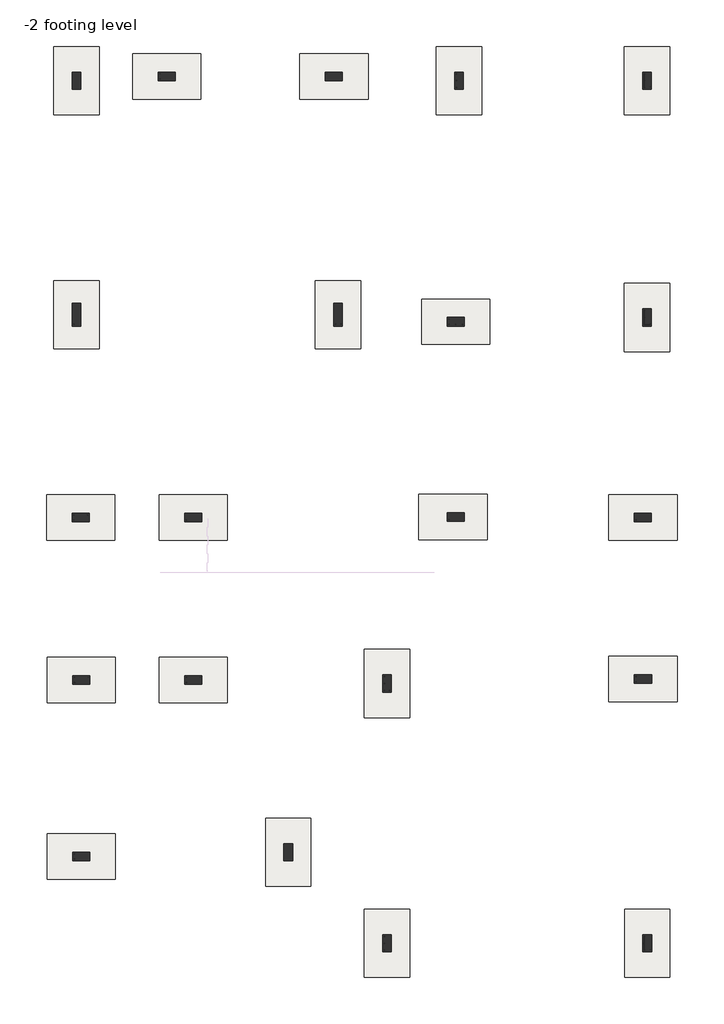
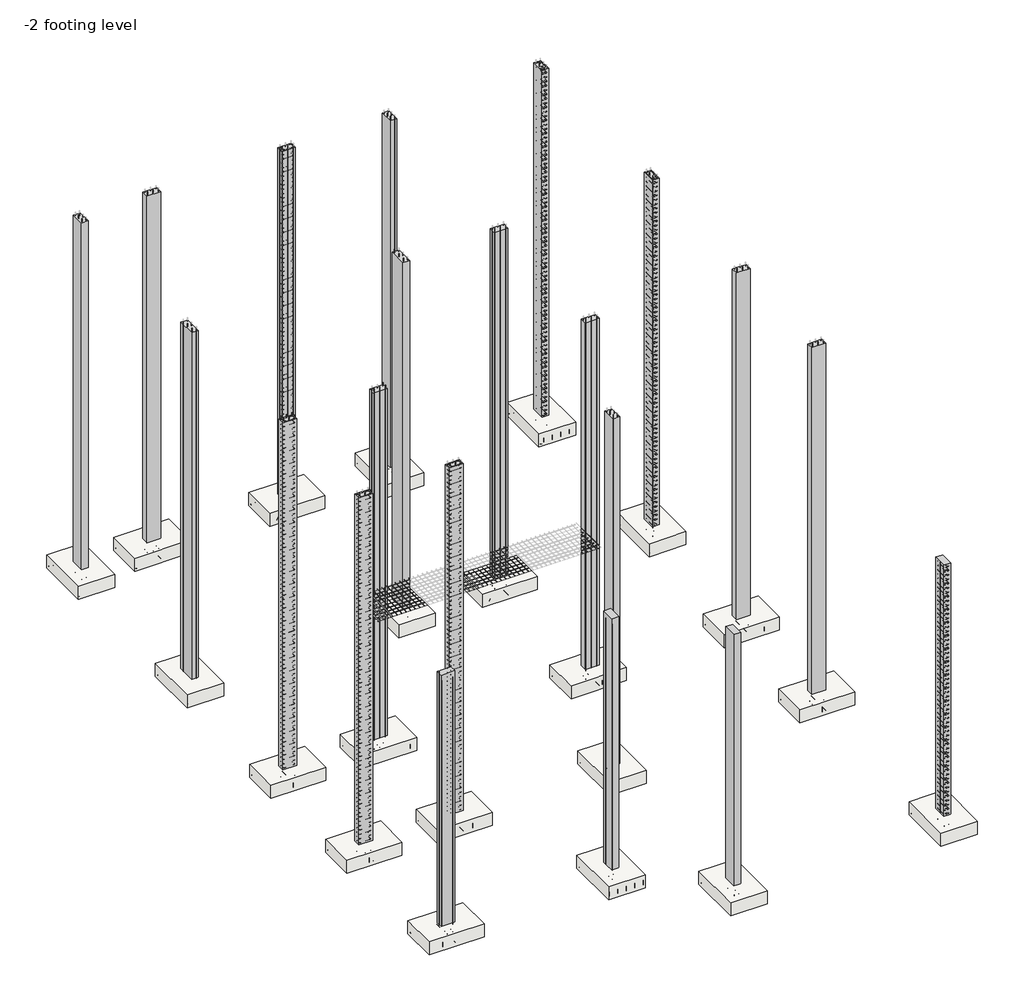
# One storey, part 1 of 9: 21 columns, 21 slabs.
"""IFC4 building model written with IfcOpenShell, lengths in millimetres."""

from ifc_helpers import new_model, si_unit, frame, origin, place, context, project, spatial, polyline, outline, extrude, faceted_brep, transform, mapped, element, save
from components import slab_5ba74754

model = new_model("IFC4")

# Units and contexts
model_context = context("Model", 3, world=origin())
ifc_project = project(units=[si_unit("LENGTHUNIT", "METRE", prefix="MILLI")], contexts=[model_context])

# Site, building, storey
site = spatial("IfcSite", under=ifc_project)
building = spatial("IfcBuilding", under=site)
storey = spatial("IfcBuildingStorey", under=building, Name="-2 footing level", Elevation=-1828.8)

# Columns
placement = place(None, origin())
element("IfcColumn", 1, ObjectType="Concrete-Rectangular-Column : 18.9", at=placement, inside=storey, context=model_context, shape_type="SweptSolid", body=[
    extrude(outline(polyline([(-8184.1001466, -7145.4266794), (-7726.9001466, -7145.4266794), (-7726.9001466, -7374.0266794), (-8184.1001466, -7374.0266794), (-8184.1001466, -7145.4266794)])), frame((0.0, 0.0, -1828.8), z_axis=(0.0, 0.0, 1.0), x_axis=(1.0, 0.0, 0.0)), (0.0, 0.0, 1.0), 8839.2),
])
element("IfcColumn", 2, ObjectType="Concrete-Rectangular-Column : 18.9", at=placement, inside=storey, context=model_context, shape_type="Brep", body=[
    faceted_brep([(-2287.8823872, -6916.8266794, -1828.8), (-2287.8823872, -7374.0266794, -1828.8), (-2516.4823872, -7374.0266794, -1828.8), (-2516.4823872, -6916.8266794, -1828.8), (-2287.8823872, -6916.8266794, 7010.4), (-2287.8823872, -7374.0266794, 7010.4), (-2287.8823872, -7374.0266794, 6553.2), (-2287.8823872, -7374.0266794, 3505.2), (-2287.8823872, -7374.0266794, 3048.0), (-2287.8823872, -6916.8266794, 3048.0), (-2287.8823872, -6916.8266794, 3505.2), (-2287.8823872, -6916.8266794, 6553.2), (-2516.4823872, -7374.0266794, 7010.4), (-2516.4823872, -7374.0266794, 6553.2), (-2516.4823872, -7374.0266794, 3505.2), (-2516.4823872, -7374.0266794, 3048.0), (-2516.4823872, -6916.8266794, 7010.4), (-2516.4823872, -6916.8266794, 6553.2), (-2516.4823872, -6916.8266794, 3505.2), (-2516.4823872, -6916.8266794, 3048.0)], [[[0, 1, 2, 3]], [[4, 5, 6, 7, 8, 1, 0, 9, 10, 11]], [[5, 12, 13, 14, 15, 2, 1, 8, 7, 6]], [[12, 16, 17, 18, 19, 3, 2, 15, 14, 13]], [[16, 4, 11, 10, 9, 0, 3, 19, 18, 17]], [[4, 16, 12, 5]]]),
])
element("IfcColumn", 3, ObjectType="Concrete-Rectangular-Column : 18.9", at=placement, inside=storey, context=model_context, shape_type="SweptSolid", body=[
    extrude(outline(polyline([(358.2588295, -9362.9794723), (358.2588295, -9820.1794723), (129.6588295, -9820.1794723), (129.6588295, -9362.9794723), (358.2588295, -9362.9794723)])), frame((0.0, 0.0, -1828.8), z_axis=(0.0, 0.0, 1.0), x_axis=(1.0, 0.0, 0.0)), (0.0, 0.0, 1.0), 8839.2),
])
element("IfcColumn", 4, ObjectType="Concrete-Rectangular-Column : 18.9", at=placement, inside=storey, context=model_context, shape_type="SweptSolid", body=[
    extrude(outline(polyline([(7338.2179176, -9362.9794723), (7338.2179176, -9820.1794723), (7109.6179176, -9820.1794723), (7109.6179176, -9362.9794723), (7338.2179176, -9362.9794723)])), frame((0.0, 0.0, -1828.8), z_axis=(0.0, 0.0, 1.0), x_axis=(1.0, 0.0, 0.0)), (0.0, 0.0, 1.0), 8839.2),
])
element("IfcColumn", 5, ObjectType="Concrete-Rectangular-Column : 18.9", at=placement, inside=storey, context=model_context, shape_type="Brep", body=[
    faceted_brep([(6881.0179176, -2394.7351307, -1828.8), (7338.2179176, -2394.7351307, -1828.8), (7338.2179176, -2623.3351307, -1828.8), (6881.0179176, -2623.3351307, -1828.8), (6881.0179176, -2394.7351307, 10363.2), (7338.2179176, -2394.7351307, 10363.2), (7338.2179176, -2394.7351307, 10058.4), (7338.2179176, -2394.7351307, 7010.4), (7338.2179176, -2394.7351307, 6553.2), (7338.2179176, -2394.7351307, 3505.2), (7338.2179176, -2394.7351307, 3048.0), (7338.2179176, -2394.7351307, 0.0), (7338.2179176, -2394.7351307, -609.6), (6881.0179176, -2394.7351307, -609.6), (6881.0179176, -2394.7351307, 0.0), (6881.0179176, -2394.7351307, 3048.0), (6881.0179176, -2394.7351307, 3505.2), (6881.0179176, -2394.7351307, 6553.2), (6881.0179176, -2394.7351307, 7010.4), (6881.0179176, -2394.7351307, 10058.4), (7338.2179176, -2623.3351307, 10363.2), (7338.2179176, -2623.3351307, 10058.4), (7338.2179176, -2623.3351307, 7010.4), (7338.2179176, -2623.3351307, 6553.2), (7338.2179176, -2623.3351307, 3505.2), (7338.2179176, -2623.3351307, 3048.0), (7338.2179176, -2623.3351307, 0.0), (7338.2179176, -2623.3351307, -609.6), (6881.0179176, -2623.3351307, 10363.2), (6881.0179176, -2623.3351307, 10058.4)], [[[0, 1, 2, 3]], [[4, 5, 6, 7, 8, 9, 10, 11, 12, 1, 0, 13, 14, 15, 16, 17, 18, 19]], [[5, 20, 21, 22, 23, 24, 25, 26, 27, 2, 1, 12, 11, 10, 9, 8, 7, 6]], [[20, 28, 29, 3, 2, 27, 26, 25, 24, 23, 22, 21]], [[28, 4, 19, 18, 17, 16, 15, 14, 13, 0, 3, 29]], [[4, 28, 20, 5]]]),
])
element("IfcColumn", 6, ObjectType="Concrete-Rectangular-Column : 18.9", at=placement, inside=storey, context=model_context, shape_type="Brep", body=[
    faceted_brep([(129.6588295, -2851.9351307, -1828.8), (129.6588295, -2394.7351307, -1828.8), (358.2588295, -2394.7351307, -1828.8), (358.2588295, -2851.9351307, -1828.8), (129.6588295, -2851.9351307, 10363.2), (129.6588295, -2394.7351307, 10363.2), (129.6588295, -2394.7351307, 10058.4), (129.6588295, -2394.7351307, 7010.4), (129.6588295, -2394.7351307, 6553.2), (129.6588295, -2394.7351307, 3505.2), (129.6588295, -2394.7351307, 3048.0), (129.6588295, -2394.7351307, 0.0), (129.6588295, -2394.7351307, -609.6), (129.6588295, -2851.9351307, -609.6), (129.6588295, -2851.9351307, 0.0), (129.6588295, -2851.9351307, 3048.0), (129.6588295, -2851.9351307, 3505.2), (129.6588295, -2851.9351307, 6553.2), (129.6588295, -2851.9351307, 7010.4), (129.6588295, -2851.9351307, 10058.4), (358.2588295, -2394.7351307, 10363.2), (358.2588295, -2394.7351307, 10058.4), (358.2588295, -2394.7351307, 7010.4), (358.2588295, -2394.7351307, 6553.2), (358.2588295, -2394.7351307, 3505.2), (358.2588295, -2394.7351307, 3048.0), (358.2588295, -2394.7351307, 0.0), (358.2588295, -2394.7351307, -609.6), (358.2588295, -2851.9351307, 10363.2), (358.2588295, -2851.9351307, 10058.4), (358.2588295, -2851.9351307, 7010.4), (358.2588295, -2851.9351307, 6553.2), (358.2588295, -2851.9351307, 3505.2), (358.2588295, -2851.9351307, 3048.0), (358.2588295, -2851.9351307, 0.0), (358.2588295, -2851.9351307, -609.6)], [[[0, 1, 2, 3]], [[4, 5, 6, 7, 8, 9, 10, 11, 12, 1, 0, 13, 14, 15, 16, 17, 18, 19]], [[5, 20, 21, 22, 23, 24, 25, 26, 27, 2, 1, 12, 11, 10, 9, 8, 7, 6]], [[20, 28, 29, 30, 31, 32, 33, 34, 35, 3, 2, 27, 26, 25, 24, 23, 22, 21]], [[28, 4, 19, 18, 17, 16, 15, 14, 13, 0, 3, 35, 34, 33, 32, 31, 30, 29]], [[4, 28, 20, 5]]]),
])
element("IfcColumn", 7, ObjectType="Concrete-Rectangular-Column : 18.9", at=placement, inside=storey, context=model_context, shape_type="Brep", body=[
    faceted_brep([(-4721.8698352, -2640.4945725, -1828.8), (-5179.0698352, -2640.4945725, -1828.8), (-5179.0698352, -2411.8945725, -1828.8), (-4721.8698352, -2411.8945725, -1828.8), (-4721.8698352, -2640.4945725, 10363.2), (-5179.0698352, -2640.4945725, 10363.2), (-5179.0698352, -2640.4945725, 10058.4), (-5179.0698352, -2640.4945725, 7010.4), (-5179.0698352, -2640.4945725, 6553.2), (-5179.0698352, -2640.4945725, 3505.2), (-5179.0698352, -2640.4945725, 3048.0), (-5179.0698352, -2640.4945725, 0.0), (-5179.0698352, -2640.4945725, -609.6), (-4721.8698352, -2640.4945725, -609.6), (-4721.8698352, -2640.4945725, 0.0), (-4721.8698352, -2640.4945725, 3048.0), (-4721.8698352, -2640.4945725, 3505.2), (-4721.8698352, -2640.4945725, 6553.2), (-4721.8698352, -2640.4945725, 7010.4), (-4721.8698352, -2640.4945725, 10058.4), (-5179.0698352, -2411.8945725, 10363.2), (-5179.0698352, -2411.8945725, 10058.4), (-5179.0698352, -2411.8945725, 7010.4), (-5179.0698352, -2411.8945725, 6553.2), (-5179.0698352, -2411.8945725, 3505.2), (-5179.0698352, -2411.8945725, 3048.0), (-5179.0698352, -2411.8945725, 0.0), (-5179.0698352, -2411.8945725, -609.6), (-4721.8698352, -2411.8945725, 10363.2), (-4721.8698352, -2411.8945725, 10058.4), (-4721.8698352, -2411.8945725, 7010.4), (-4721.8698352, -2411.8945725, 6553.2), (-4721.8698352, -2411.8945725, 3505.2), (-4721.8698352, -2411.8945725, 3048.0), (-4721.8698352, -2411.8945725, 0.0), (-4721.8698352, -2411.8945725, -609.6)], [[[0, 1, 2, 3]], [[4, 5, 6, 7, 8, 9, 10, 11, 12, 1, 0, 13, 14, 15, 16, 17, 18, 19]], [[5, 20, 21, 22, 23, 24, 25, 26, 27, 2, 1, 12, 11, 10, 9, 8, 7, 6]], [[20, 28, 29, 30, 31, 32, 33, 34, 35, 3, 2, 27, 26, 25, 24, 23, 22, 21]], [[28, 4, 19, 18, 17, 16, 15, 14, 13, 0, 3, 35, 34, 33, 32, 31, 30, 29]], [[4, 28, 20, 5]]]),
])
element("IfcColumn", 8, ObjectType="Concrete-Rectangular-Column : 18.9", at=placement, inside=storey, context=model_context, shape_type="Brep", body=[
    faceted_brep([(-7726.9001466, -2640.4945725, -1828.8), (-8184.1001466, -2640.4945725, -1828.8), (-8184.1001466, -2411.8945725, -1828.8), (-7726.9001466, -2411.8945725, -1828.8), (-7726.9001466, -2640.4945725, 10363.2), (-8184.1001466, -2640.4945725, 10363.2), (-8184.1001466, -2640.4945725, 10058.4), (-8184.1001466, -2640.4945725, 7010.4), (-8184.1001466, -2640.4945725, 6553.2), (-8184.1001466, -2640.4945725, 3505.2), (-8184.1001466, -2640.4945725, 3048.0), (-7726.9001466, -2640.4945725, 3048.0), (-7726.9001466, -2640.4945725, 3505.2), (-7726.9001466, -2640.4945725, 6553.2), (-7726.9001466, -2640.4945725, 7010.4), (-7726.9001466, -2640.4945725, 10058.4), (-8184.1001466, -2411.8945725, 10363.2), (-8184.1001466, -2411.8945725, 10058.4), (-8184.1001466, -2411.8945725, 7010.4), (-8184.1001466, -2411.8945725, 6553.2), (-8184.1001466, -2411.8945725, 3505.2), (-8184.1001466, -2411.8945725, 3048.0), (-7726.9001466, -2411.8945725, 10363.2), (-7726.9001466, -2411.8945725, 10058.4), (-7726.9001466, -2411.8945725, 7010.4), (-7726.9001466, -2411.8945725, 6553.2), (-7726.9001466, -2411.8945725, 3505.2), (-7726.9001466, -2411.8945725, 3048.0)], [[[0, 1, 2, 3]], [[4, 5, 6, 7, 8, 9, 10, 1, 0, 11, 12, 13, 14, 15]], [[5, 16, 17, 18, 19, 20, 21, 2, 1, 10, 9, 8, 7, 6]], [[16, 22, 23, 24, 25, 26, 27, 3, 2, 21, 20, 19, 18, 17]], [[22, 4, 15, 14, 13, 12, 11, 0, 3, 27, 26, 25, 24, 23]], [[4, 22, 16, 5]]]),
])
element("IfcColumn", 9, ObjectType="Concrete-Rectangular-Column : 18.9", at=placement, inside=storey, context=model_context, shape_type="Brep", body=[
    faceted_brep([(-4722.5687565, 1710.0401753, -1828.8), (-5179.7687565, 1710.0401753, -1828.8), (-5179.7687565, 1938.6401753, -1828.8), (-4722.5687565, 1938.6401753, -1828.8), (-4722.5687565, 1710.0401753, 10363.2), (-5179.0698352, 1710.0401753, 10363.2), (-5179.7687565, 1710.0401753, 10363.2), (-4722.5687565, 1710.0401753, 10058.4), (-5179.7687565, 1722.9180142, 10363.2), (-5179.7687565, 1938.6401753, 10363.2), (-5179.7687565, 1938.6401753, 10058.4), (-5179.7687565, 1938.6401753, 7010.4), (-5179.7687565, 1938.6401753, 6553.2), (-5179.7687565, 1938.6401753, 3505.2), (-5179.7687565, 1938.6401753, 3048.0), (-5179.7687565, 1938.6401753, 0.0), (-5179.7687565, 1938.6401753, -609.6), (-4722.5687565, 1938.6401753, 10363.2), (-4722.5687565, 1938.6401753, 10058.4), (-4722.5687565, 1938.6401753, 7010.4), (-4722.5687565, 1938.6401753, 6553.2), (-4722.5687565, 1938.6401753, 3505.2), (-4722.5687565, 1938.6401753, 3048.0), (-4722.5687565, 1938.6401753, 0.0), (-4722.5687565, 1938.6401753, -609.6), (-4722.5687565, 1722.9180142, 10363.2)], [[[0, 1, 2, 3]], [[4, 5, 6, 1, 0, 7]], [[6, 8, 9, 10, 11, 12, 13, 14, 15, 16, 2, 1]], [[9, 17, 18, 19, 20, 21, 22, 23, 24, 3, 2, 16, 15, 14, 13, 12, 11, 10]], [[17, 25, 4, 7, 0, 3, 24, 23, 22, 21, 20, 19, 18]], [[4, 25, 17, 9, 8, 6, 5]]]),
])
element("IfcColumn", 10, ObjectType="Concrete-Rectangular-Column : 18.9", at=placement, inside=storey, context=model_context, shape_type="Brep", body=[
    faceted_brep([(-7740.635762, 1710.0401753, -1828.8), (-8197.835762, 1710.0401753, -1828.8), (-8197.835762, 1938.6401753, -1828.8), (-7740.635762, 1938.6401753, -1828.8), (-7740.635762, 1710.0401753, 10363.2), (-8197.835762, 1710.0401753, 10363.2), (-8197.835762, 1710.0401753, 10058.4), (-7740.635762, 1710.0401753, 10058.4), (-8197.835762, 1938.6401753, 10363.2), (-8197.835762, 1938.6401753, 10058.4), (-7740.635762, 1938.6401753, 10363.2), (-7740.635762, 1938.6401753, 10058.4)], [[[0, 1, 2, 3]], [[4, 5, 6, 1, 0, 7]], [[5, 8, 9, 2, 1, 6]], [[8, 10, 11, 3, 2, 9]], [[10, 4, 7, 0, 3, 11]], [[4, 10, 8, 5]]]),
])
element("IfcColumn", 11, ObjectType="Concrete-Rectangular-Column : 18.9", at=placement, inside=storey, context=model_context, shape_type="Brep", body=[
    faceted_brep([(1859.2315874, 7190.7340845, -1828.8), (2316.4315874, 7190.7340845, -1828.8), (2316.4315874, 6962.1340845, -1828.8), (1859.2315874, 6962.1340845, -1828.8), (1859.2315874, 7190.7340845, 10363.2), (2316.4315874, 7190.7340845, 10363.2), (2316.4315874, 7190.7340845, 10058.4), (2316.4315874, 7190.7340845, 7010.4), (2316.4315874, 7190.7340845, 6553.2), (2316.4315874, 7190.7340845, 3505.2), (2316.4315874, 7190.7340845, 3048.0), (2316.4315874, 7190.7340845, 0.0), (2316.4315874, 7190.7340845, -609.6), (1859.2315874, 7190.7340845, -609.6), (1859.2315874, 7190.7340845, 0.0), (1859.2315874, 7190.7340845, 3048.0), (1859.2315874, 7190.7340845, 3505.2), (1859.2315874, 7190.7340845, 6553.2), (1859.2315874, 7190.7340845, 7010.4), (1859.2315874, 7190.7340845, 10058.4), (2316.4315874, 6962.1340845, 10363.2), (2316.4315874, 6962.1340845, 10058.4), (2316.4315874, 6962.1340845, 7010.4), (2316.4315874, 6962.1340845, 6553.2), (2316.4315874, 6962.1340845, 3505.2), (2316.4315874, 6962.1340845, 3048.0), (2316.4315874, 6962.1340845, 0.0), (2316.4315874, 6962.1340845, -609.6), (1859.2315874, 6962.1340845, 10363.2), (1859.2315874, 6962.1340845, 10058.4), (1859.2315874, 6962.1340845, 7010.4), (1859.2315874, 6962.1340845, 6553.2), (1859.2315874, 6962.1340845, 3505.2), (1859.2315874, 6962.1340845, 3048.0), (1859.2315874, 6962.1340845, 0.0), (1859.2315874, 6962.1340845, -609.6)], [[[0, 1, 2, 3]], [[4, 5, 6, 7, 8, 9, 10, 11, 12, 1, 0, 13, 14, 15, 16, 17, 18, 19]], [[5, 20, 21, 22, 23, 24, 25, 26, 27, 2, 1, 12, 11, 10, 9, 8, 7, 6]], [[20, 28, 29, 30, 31, 32, 33, 34, 35, 3, 2, 27, 26, 25, 24, 23, 22, 21]], [[28, 4, 19, 18, 17, 16, 15, 14, 13, 0, 3, 35, 34, 33, 32, 31, 30, 29]], [[4, 28, 20, 5]]]),
])
element("IfcColumn", 12, ObjectType="Concrete-Rectangular-Column : 18.9", at=placement, inside=storey, context=model_context, shape_type="Brep", body=[
    faceted_brep([(7108.8638577, 6962.1340845, -1828.8), (7108.8638577, 7419.3340845, -1828.8), (7337.4638577, 7419.3340845, -1828.8), (7337.4638577, 6962.1340845, -1828.8), (7108.8638577, 6962.1340845, 10363.2), (7108.8638577, 7419.3340845, 10363.2), (7108.8638577, 7419.3340845, 10058.4), (7108.8638577, 6962.1340845, 10058.4), (7337.4638577, 7419.3340845, 10363.2), (7337.4638577, 7419.3340845, 10058.4), (7337.4638577, 6962.1340845, 10363.2), (7337.4638577, 6962.1340845, 10058.4)], [[[0, 1, 2, 3]], [[4, 5, 6, 1, 0, 7]], [[5, 8, 9, 2, 1, 6]], [[8, 10, 11, 3, 2, 9]], [[10, 4, 7, 0, 3, 11]], [[4, 10, 8, 5]]]),
])
element("IfcColumn", 13, ObjectType="Concrete-Rectangular-Column : 18.9", at=placement, inside=storey, context=model_context, shape_type="Brep", body=[
    faceted_brep([(2316.4315874, 1722.9180142, -1828.8), (1859.2315874, 1722.9180142, -1828.8), (1859.2315874, 1951.5180142, -1828.8), (2316.4315874, 1951.5180142, -1828.8), (2316.4315874, 1722.9180142, 10363.2), (1859.2315874, 1722.9180142, 10363.2), (1859.2315874, 1722.9180142, 10058.4), (1859.2315874, 1722.9180142, 7010.4), (1859.2315874, 1722.9180142, 6553.2), (1859.2315874, 1722.9180142, 3505.2), (1859.2315874, 1722.9180142, 3048.0), (1859.2315874, 1722.9180142, 0.0), (1859.2315874, 1722.9180142, -609.6), (2316.4315874, 1722.9180142, -609.6), (2316.4315874, 1722.9180142, 0.0), (2316.4315874, 1722.9180142, 3048.0), (2316.4315874, 1722.9180142, 3505.2), (2316.4315874, 1722.9180142, 6553.2), (2316.4315874, 1722.9180142, 7010.4), (2316.4315874, 1722.9180142, 10058.4), (1859.2315874, 1951.5180142, 10363.2), (1859.2315874, 1951.5180142, 10058.4), (1859.2315874, 1951.5180142, 7010.4), (1859.2315874, 1951.5180142, 6553.2), (1859.2315874, 1951.5180142, 3505.2), (1859.2315874, 1951.5180142, 3048.0), (1859.2315874, 1951.5180142, 0.0), (1859.2315874, 1951.5180142, -609.6), (2316.4315874, 1951.5180142, 10363.2), (2316.4315874, 1951.5180142, 10058.4), (2316.4315874, 1951.5180142, 7010.4), (2316.4315874, 1951.5180142, 6553.2), (2316.4315874, 1951.5180142, 3505.2), (2316.4315874, 1951.5180142, 3048.0), (2316.4315874, 1951.5180142, 0.0), (2316.4315874, 1951.5180142, -609.6)], [[[0, 1, 2, 3]], [[4, 5, 6, 7, 8, 9, 10, 11, 12, 1, 0, 13, 14, 15, 16, 17, 18, 19]], [[5, 20, 21, 22, 23, 24, 25, 26, 27, 2, 1, 12, 11, 10, 9, 8, 7, 6]], [[20, 28, 29, 30, 31, 32, 33, 34, 35, 3, 2, 27, 26, 25, 24, 23, 22, 21]], [[28, 4, 19, 18, 17, 16, 15, 14, 13, 0, 3, 35, 34, 33, 32, 31, 30, 29]], [[4, 28, 20, 5]]]),
])
element("IfcColumn", 14, ObjectType="Concrete-Rectangular-Column : 18.9", at=placement, inside=storey, context=model_context, shape_type="Brep", body=[
    faceted_brep([(7336.8310303, 1718.3038411, -1828.8), (6879.6310303, 1718.3038411, -1828.8), (6879.6310303, 1946.9038411, -1828.8), (7336.8310303, 1946.9038411, -1828.8), (7336.8310303, 1718.3038411, 10363.2), (6994.5638577, 1718.3038411, 10363.2), (6879.6310303, 1718.3038411, 10363.2), (7336.8310303, 1718.3038411, -609.6), (7336.8310303, 1718.3038411, 0.0), (7336.8310303, 1718.3038411, 3048.0), (7336.8310303, 1718.3038411, 3505.2), (7336.8310303, 1718.3038411, 6553.2), (7336.8310303, 1718.3038411, 7010.4), (7336.8310303, 1718.3038411, 10058.4), (6879.6310303, 1722.9180142, 10363.2), (6879.6310303, 1946.9038411, 10363.2), (6879.6310303, 1946.9038411, 10058.4), (6994.5638577, 1946.9038411, 10363.2), (7336.8310303, 1946.9038411, 10363.2), (7336.8310303, 1946.9038411, 10058.4), (7336.8310303, 1946.9038411, 7010.4), (7336.8310303, 1946.9038411, 6553.2), (7336.8310303, 1946.9038411, 3505.2), (7336.8310303, 1946.9038411, 3048.0), (7336.8310303, 1946.9038411, 0.0), (7336.8310303, 1946.9038411, -609.6)], [[[0, 1, 2, 3]], [[4, 5, 6, 1, 0, 7, 8, 9, 10, 11, 12, 13]], [[6, 14, 15, 16, 2, 1]], [[15, 17, 18, 19, 20, 21, 22, 23, 24, 25, 3, 2, 16]], [[18, 4, 13, 12, 11, 10, 9, 8, 7, 0, 3, 25, 24, 23, 22, 21, 20, 19]], [[4, 18, 17, 15, 14, 6, 5]]]),
])
element("IfcColumn", 15, ObjectType="Concrete-Rectangular-Column : 18.9", at=placement, inside=storey, context=model_context, shape_type="Brep", body=[
    faceted_brep([(2290.2821988, 13770.1951007, -1828.8), (2290.2821988, 13312.9951007, -1828.8), (2061.6821988, 13312.9951007, -1828.8), (2061.6821988, 13770.1951007, -1828.8), (2290.2821988, 13770.1951007, 10363.2), (2290.2821988, 13312.9951007, 10363.2), (2290.2821988, 13312.9951007, 10058.4), (2290.2821988, 13312.9951007, 7010.4), (2290.2821988, 13312.9951007, 6553.2), (2290.2821988, 13312.9951007, 3505.2), (2290.2821988, 13312.9951007, 3048.0), (2290.2821988, 13312.9951007, 0.0), (2290.2821988, 13312.9951007, -609.6), (2290.2821988, 13770.1951007, -609.6), (2290.2821988, 13770.1951007, 0.0), (2290.2821988, 13770.1951007, 3048.0), (2290.2821988, 13770.1951007, 3505.2), (2290.2821988, 13770.1951007, 6553.2), (2290.2821988, 13770.1951007, 7010.4), (2290.2821988, 13770.1951007, 10058.4), (2061.6821988, 13312.9951007, 10363.2), (2061.6821988, 13312.9951007, 10058.4), (2061.6821988, 13312.9951007, 7010.4), (2061.6821988, 13312.9951007, 6553.2), (2061.6821988, 13312.9951007, 3505.2), (2061.6821988, 13312.9951007, 3048.0), (2061.6821988, 13312.9951007, 0.0), (2061.6821988, 13312.9951007, -609.6), (2061.6821988, 13770.1951007, 10363.2), (2061.6821988, 13770.1951007, 10058.4), (2061.6821988, 13770.1951007, 7010.4), (2061.6821988, 13770.1951007, 6553.2), (2061.6821988, 13770.1951007, 3505.2), (2061.6821988, 13770.1951007, 3048.0), (2061.6821988, 13770.1951007, 0.0), (2061.6821988, 13770.1951007, -609.6)], [[[0, 1, 2, 3]], [[4, 5, 6, 7, 8, 9, 10, 11, 12, 1, 0, 13, 14, 15, 16, 17, 18, 19]], [[5, 20, 21, 22, 23, 24, 25, 26, 27, 2, 1, 12, 11, 10, 9, 8, 7, 6]], [[20, 28, 29, 30, 31, 32, 33, 34, 35, 3, 2, 27, 26, 25, 24, 23, 22, 21]], [[28, 4, 19, 18, 17, 16, 15, 14, 13, 0, 3, 35, 34, 33, 32, 31, 30, 29]], [[4, 28, 20, 5]]]),
])
element("IfcColumn", 16, ObjectType="Concrete-Rectangular-Column : 18.9", at=placement, inside=storey, context=model_context, shape_type="Brep", body=[
    faceted_brep([(7337.4638577, 13770.1951007, -1828.8), (7337.4638577, 13312.9951007, -1828.8), (7108.8638577, 13312.9951007, -1828.8), (7108.8638577, 13770.1951007, -1828.8), (7337.4638577, 13770.1951007, 10363.2), (7337.4638577, 13312.9951007, 10363.2), (7337.4638577, 13312.9951007, 10058.4), (7337.4638577, 13770.1951007, 10058.4), (7108.8638577, 13312.9951007, 10363.2), (7108.8638577, 13312.9951007, 10058.4), (7108.8638577, 13770.1951007, 10363.2), (7108.8638577, 13770.1951007, 10058.4)], [[[0, 1, 2, 3]], [[4, 5, 6, 1, 0, 7]], [[5, 8, 9, 2, 1, 6]], [[8, 10, 11, 3, 2, 9]], [[10, 4, 7, 0, 3, 11]], [[4, 10, 8, 5]]]),
])
element("IfcColumn", 17, ObjectType="Concrete-Rectangular-Column : 18.9", at=placement, inside=storey, context=model_context, shape_type="Brep", body=[
    faceted_brep([(-1405.4178012, 13770.1951007, -1828.8), (-948.2178012, 13770.1951007, -1828.8), (-948.2178012, 13541.5951007, -1828.8), (-1405.4178012, 13541.5951007, -1828.8), (-1405.4178012, 13770.1951007, 10363.2), (-948.2178012, 13770.1951007, 10363.2), (-948.2178012, 13770.1951007, 10058.4), (-948.2178012, 13770.1951007, 7010.4), (-948.2178012, 13770.1951007, 6553.2), (-948.2178012, 13770.1951007, 3505.2), (-948.2178012, 13770.1951007, 3048.0), (-948.2178012, 13770.1951007, 0.0), (-948.2178012, 13770.1951007, -609.6), (-1405.4178012, 13770.1951007, -609.6), (-1405.4178012, 13770.1951007, 0.0), (-1405.4178012, 13770.1951007, 3048.0), (-1405.4178012, 13770.1951007, 3505.2), (-1405.4178012, 13770.1951007, 6553.2), (-1405.4178012, 13770.1951007, 7010.4), (-1405.4178012, 13770.1951007, 10058.4), (-948.2178012, 13541.5951007, 10363.2), (-948.2178012, 13541.5951007, 10058.4), (-948.2178012, 13541.5951007, 7010.4), (-948.2178012, 13541.5951007, 6553.2), (-948.2178012, 13541.5951007, 3505.2), (-948.2178012, 13541.5951007, 3048.0), (-948.2178012, 13541.5951007, 0.0), (-948.2178012, 13541.5951007, -609.6), (-1405.4178012, 13541.5951007, 10363.2), (-1405.4178012, 13541.5951007, 10058.4), (-1405.4178012, 13541.5951007, 7010.4), (-1405.4178012, 13541.5951007, 6553.2), (-1405.4178012, 13541.5951007, 3505.2), (-1405.4178012, 13541.5951007, 3048.0), (-1405.4178012, 13541.5951007, 0.0), (-1405.4178012, 13541.5951007, -609.6)], [[[0, 1, 2, 3]], [[4, 5, 6, 7, 8, 9, 10, 11, 12, 1, 0, 13, 14, 15, 16, 17, 18, 19]], [[5, 20, 21, 22, 23, 24, 25, 26, 27, 2, 1, 12, 11, 10, 9, 8, 7, 6]], [[20, 28, 29, 30, 31, 32, 33, 34, 35, 3, 2, 27, 26, 25, 24, 23, 22, 21]], [[28, 4, 19, 18, 17, 16, 15, 14, 13, 0, 3, 35, 34, 33, 32, 31, 30, 29]], [[4, 28, 20, 5]]]),
])
element("IfcColumn", 18, ObjectType="Concrete-Rectangular-Column : 18.9", at=placement, inside=storey, context=model_context, shape_type="Brep", body=[
    faceted_brep([(-5887.9819615, 13770.1951007, -1828.8), (-5430.7819615, 13770.1951007, -1828.8), (-5430.7819615, 13541.5951007, -1828.8), (-5887.9819615, 13541.5951007, -1828.8), (-5887.9819615, 13770.1951007, 10363.2), (-5430.7819615, 13770.1951007, 10363.2), (-5430.7819615, 13770.1951007, 10058.4), (-5430.7819615, 13770.1951007, 7010.4), (-5430.7819615, 13770.1951007, 6553.2), (-5430.7819615, 13770.1951007, 3352.8), (-5430.7819615, 13770.1951007, 3048.0), (-5430.7819615, 13770.1951007, 0.0), (-5430.7819615, 13770.1951007, -609.6), (-5887.9819615, 13770.1951007, -609.6), (-5887.9819615, 13770.1951007, 0.0), (-5887.9819615, 13770.1951007, 3048.0), (-5887.9819615, 13770.1951007, 3352.8), (-5887.9819615, 13770.1951007, 6553.2), (-5887.9819615, 13770.1951007, 7010.4), (-5887.9819615, 13770.1951007, 10058.4), (-5430.7819615, 13541.5951007, 10363.2), (-5430.7819615, 13541.5951007, 10058.4), (-5430.7819615, 13541.5951007, 7010.4), (-5430.7819615, 13541.5951007, 6553.2), (-5430.7819615, 13541.5951007, 3352.8), (-5430.7819615, 13541.5951007, 3048.0), (-5430.7819615, 13541.5951007, 0.0), (-5430.7819615, 13541.5951007, -609.6), (-5887.9819615, 13541.5951007, 10363.2), (-5887.9819615, 13541.5951007, 10058.4), (-5887.9819615, 13541.5951007, 7010.4), (-5887.9819615, 13541.5951007, 6553.2), (-5887.9819615, 13541.5951007, 3352.8), (-5887.9819615, 13541.5951007, 3048.0), (-5887.9819615, 13541.5951007, 0.0), (-5887.9819615, 13541.5951007, -609.6)], [[[0, 1, 2, 3]], [[4, 5, 6, 7, 8, 9, 10, 11, 12, 1, 0, 13, 14, 15, 16, 17, 18, 19]], [[5, 20, 21, 22, 23, 24, 25, 26, 27, 2, 1, 12, 11, 10, 9, 8, 7, 6]], [[20, 28, 29, 30, 31, 32, 33, 34, 35, 3, 2, 27, 26, 25, 24, 23, 22, 21]], [[28, 4, 19, 18, 17, 16, 15, 14, 13, 0, 3, 35, 34, 33, 32, 31, 30, 29]], [[4, 28, 20, 5]]]),
])
element("IfcColumn", 19, ObjectType="Concrete-Rectangular-Column : 18.9", at=placement, inside=storey, context=model_context, shape_type="Brep", body=[
    faceted_brep([(-8197.835762, 13312.9951007, -1828.8), (-8197.835762, 13770.1951007, -1828.8), (-7969.235762, 13770.1951007, -1828.8), (-7969.235762, 13312.9951007, -1828.8), (-8197.835762, 13312.9951007, 10363.2), (-8197.835762, 13770.1951007, 10363.2), (-8197.835762, 13312.9951007, 10058.4), (-7969.235762, 13770.1951007, 10363.2), (-7969.235762, 13770.1951007, 10058.4), (-7969.235762, 13312.9951007, 10363.2), (-7969.235762, 13312.9951007, 10058.4)], [[[0, 1, 2, 3]], [[4, 5, 1, 0, 6]], [[5, 7, 8, 2, 1]], [[7, 9, 10, 3, 2, 8]], [[9, 4, 6, 0, 3, 10]], [[4, 9, 7, 5]]]),
])
element("IfcColumn", 20, ObjectType="Concrete-Rectangular-Column : 2.9", at=placement, inside=storey, context=model_context, shape_type="Brep", body=[
    faceted_brep([(-7972.3115433, 7571.2780739, -1828.8), (-7972.3115433, 6961.6780739, -1828.8), (-8200.9115433, 6961.6780739, -1828.8), (-8200.9115433, 7571.2780739, -1828.8), (-7972.3115433, 7571.2780739, 10363.2), (-7972.3115433, 6961.6780739, 10363.2), (-7972.3115433, 6961.6780739, 10058.4), (-7972.3115433, 6961.6780739, 7010.4), (-7972.3115433, 6961.6780739, 6553.2), (-7972.3115433, 6961.6780739, 3505.2), (-7972.3115433, 6961.6780739, 3048.0), (-7972.3115433, 6961.6780739, 0.0), (-7972.3115433, 6961.6780739, -609.6), (-7972.3115433, 7571.2780739, -609.6), (-7972.3115433, 7571.2780739, 0.0), (-7972.3115433, 7571.2780739, 3048.0), (-7972.3115433, 7571.2780739, 3352.8), (-7972.3115433, 7571.2780739, 6553.2), (-7972.3115433, 7571.2780739, 7010.4), (-7972.3115433, 7571.2780739, 10058.4), (-8197.835762, 6961.6780739, 10363.2), (-8200.9115433, 6961.6780739, 10363.2), (-8200.9115433, 7571.2780739, 10363.2), (-8197.835762, 7571.2780739, 10363.2)], [[[0, 1, 2, 3]], [[4, 5, 6, 7, 8, 9, 10, 11, 12, 1, 0, 13, 14, 15, 16, 17, 18, 19]], [[5, 20, 21, 2, 1, 12, 11, 10, 9, 8, 7, 6]], [[21, 22, 3, 2]], [[22, 23, 4, 19, 18, 17, 16, 15, 14, 13, 0, 3]], [[4, 23, 22, 21, 20, 5]]]),
])
element("IfcColumn", 21, ObjectType="Concrete-Rectangular-Column : 2.9", at=placement, inside=storey, context=model_context, shape_type="Brep", body=[
    faceted_brep([(-948.2178012, 7571.7340845, -1828.8), (-948.2178012, 6962.1340845, -1828.8), (-1176.8178012, 6962.1340845, -1828.8), (-1176.8178012, 7571.7340845, -1828.8), (-948.2178012, 7571.7340845, 10363.2), (-948.2178012, 7419.3340845, 10363.2), (-948.2178012, 6962.1340845, 10363.2), (-948.2178012, 6962.1340845, 10058.4), (-948.2178012, 6962.1340845, 7010.4), (-948.2178012, 6962.1340845, 6553.2), (-948.2178012, 6962.1340845, 3505.2), (-948.2178012, 6962.1340845, 3048.0), (-948.2178012, 6962.1340845, 0.0), (-948.2178012, 6962.1340845, -609.6), (-948.2178012, 7571.7340845, 10058.4), (-1176.8178012, 6962.1340845, 10363.2), (-1176.8178012, 6962.1340845, 10058.4), (-1176.8178012, 6962.1340845, 7010.4), (-1176.8178012, 6962.1340845, 6553.2), (-1176.8178012, 6962.1340845, 3505.2), (-1176.8178012, 6962.1340845, 3048.0), (-1176.8178012, 6962.1340845, 0.0), (-1176.8178012, 6962.1340845, -609.6), (-1176.8178012, 7419.3340845, 10363.2), (-1176.8178012, 7571.7340845, 10363.2), (-1176.8178012, 7571.7340845, 10058.4)], [[[0, 1, 2, 3]], [[4, 5, 6, 7, 8, 9, 10, 11, 12, 13, 1, 0, 14]], [[6, 15, 16, 17, 18, 19, 20, 21, 22, 2, 1, 13, 12, 11, 10, 9, 8, 7]], [[15, 23, 24, 25, 3, 2, 22, 21, 20, 19, 18, 17, 16]], [[24, 4, 14, 0, 3, 25]], [[4, 24, 23, 15, 6, 5]]]),
])

# Slabs
slab_shape = slab_5ba74754(model_context)
element("IfcSlab", 22, ObjectType="Footing-Rectangular : 72\" x 48\" x 18\"", at=placement, inside=storey, context=model_context, shape_type="MappedRepresentation", body=[
    mapped(slab_shape, transform((-7955.5001466, -7259.7266794, -1828.8), x_axis=(0.0, 1.0, 0.0), y_axis=(-1.0, 0.0, 0.0), z_axis=(0.0, 0.0, 1.0))),
])
element("IfcSlab", 23, ObjectType="Footing-Rectangular : 72\" x 48\" x 18\"", at=placement, inside=storey, context=model_context, shape_type="MappedRepresentation", body=[
    mapped(slab_shape, transform((-2402.1823872, -7145.4266794, -1828.8), x_axis=(1.0, 0.0, 0.0), y_axis=(0.0, 1.0, 0.0), z_axis=(0.0, 0.0, 1.0))),
])
element("IfcSlab", 24, ObjectType="Footing-Rectangular : 72\" x 48\" x 18\"", at=placement, inside=storey, context=model_context, shape_type="MappedRepresentation", body=[
    mapped(slab_shape, transform((243.9588295, -9591.5794723, -1828.8), x_axis=(1.0, 0.0, 0.0), y_axis=(0.0, 1.0, 0.0), z_axis=(0.0, 0.0, 1.0))),
])
element("IfcSlab", 25, ObjectType="Footing-Rectangular : 72\" x 48\" x 18\"", at=placement, inside=storey, context=model_context, shape_type="MappedRepresentation", body=[
    mapped(slab_shape, transform((7223.9179176, -9591.5794723, -1828.8), x_axis=(1.0, 0.0, 0.0), y_axis=(0.0, 1.0, 0.0), z_axis=(0.0, 0.0, 1.0))),
])
element("IfcSlab", 26, ObjectType="Footing-Rectangular : 72\" x 48\" x 18\"", at=placement, inside=storey, context=model_context, shape_type="MappedRepresentation", body=[
    mapped(slab_shape, transform((7109.6179176, -2509.0351307, -1828.8), x_axis=(0.0, 1.0, 0.0), y_axis=(-1.0, 0.0, 0.0), z_axis=(0.0, 0.0, 1.0))),
])
element("IfcSlab", 27, ObjectType="Footing-Rectangular : 72\" x 48\" x 18\"", at=placement, inside=storey, context=model_context, shape_type="MappedRepresentation", body=[
    mapped(slab_shape, transform((243.9588295, -2623.3351307, -1828.8), x_axis=(-1.0, 0.0, 0.0), y_axis=(0.0, -1.0, 0.0), z_axis=(0.0, 0.0, 1.0))),
])
element("IfcSlab", 28, ObjectType="Footing-Rectangular : 72\" x 48\" x 18\"", at=placement, inside=storey, context=model_context, shape_type="MappedRepresentation", body=[
    mapped(slab_shape, transform((-4950.4698352, -2526.1945725, -1828.8), x_axis=(0.0, -1.0, 0.0), y_axis=(1.0, 0.0, 0.0), z_axis=(0.0, 0.0, 1.0))),
])
element("IfcSlab", 29, ObjectType="Footing-Rectangular : 72\" x 48\" x 18\"", at=placement, inside=storey, context=model_context, shape_type="MappedRepresentation", body=[
    mapped(slab_shape, transform((-7955.5001466, -2526.1945725, -1828.8), x_axis=(0.0, -1.0, 0.0), y_axis=(1.0, 0.0, 0.0), z_axis=(0.0, 0.0, 1.0))),
])
element("IfcSlab", 30, ObjectType="Footing-Rectangular : 72\" x 48\" x 18\"", at=placement, inside=storey, context=model_context, shape_type="MappedRepresentation", body=[
    mapped(slab_shape, transform((-4951.1687565, 1824.3401753, -1828.8), x_axis=(0.0, -1.0, 0.0), y_axis=(1.0, 0.0, 0.0), z_axis=(0.0, 0.0, 1.0))),
])
element("IfcSlab", 31, ObjectType="Footing-Rectangular : 72\" x 48\" x 18\"", at=placement, inside=storey, context=model_context, shape_type="MappedRepresentation", body=[
    mapped(slab_shape, transform((-7969.235762, 1824.3401753, -1828.8), x_axis=(0.0, -1.0, 0.0), y_axis=(1.0, 0.0, 0.0), z_axis=(0.0, 0.0, 1.0))),
])
element("IfcSlab", 32, ObjectType="Footing-Rectangular : 72\" x 48\" x 18\"", at=placement, inside=storey, context=model_context, shape_type="MappedRepresentation", body=[
    mapped(slab_shape, transform((-8086.6115433, 7266.4780739, -1828.8), x_axis=(1.0, 0.0, 0.0), y_axis=(0.0, 1.0, 0.0), z_axis=(0.0, 0.0, 1.0))),
])
element("IfcSlab", 33, ObjectType="Footing-Rectangular : 72\" x 48\" x 18\"", at=placement, inside=storey, context=model_context, shape_type="MappedRepresentation", body=[
    mapped(slab_shape, transform((-1062.5178012, 7266.9340845, -1828.8), x_axis=(1.0, 0.0, 0.0), y_axis=(0.0, 1.0, 0.0), z_axis=(0.0, 0.0, 1.0))),
])
element("IfcSlab", 34, ObjectType="Footing-Rectangular : 72\" x 48\" x 18\"", at=placement, inside=storey, context=model_context, shape_type="MappedRepresentation", body=[
    mapped(slab_shape, transform((2087.8315874, 7076.4340845, -1828.8), x_axis=(0.0, 1.0, 0.0), y_axis=(-1.0, 0.0, 0.0), z_axis=(0.0, 0.0, 1.0))),
])
element("IfcSlab", 35, ObjectType="Footing-Rectangular : 72\" x 48\" x 18\"", at=placement, inside=storey, context=model_context, shape_type="MappedRepresentation", body=[
    mapped(slab_shape, transform((7223.1638577, 7190.7340845, -1828.8), x_axis=(-1.0, 0.0, 0.0), y_axis=(0.0, -1.0, 0.0), z_axis=(0.0, 0.0, 1.0))),
])
element("IfcSlab", 36, ObjectType="Footing-Rectangular : 72\" x 48\" x 18\"", at=placement, inside=storey, context=model_context, shape_type="MappedRepresentation", body=[
    mapped(slab_shape, transform((2017.4215337, 1837.2180142, -1828.8), x_axis=(0.0, -1.0, 0.0), y_axis=(1.0, 0.0, 0.0), z_axis=(0.0, 0.0, 1.0))),
])
element("IfcSlab", 37, ObjectType="Footing-Rectangular : 72\" x 48\" x 18\"", at=placement, inside=storey, context=model_context, shape_type="MappedRepresentation", body=[
    mapped(slab_shape, transform((7108.2310303, 1832.6038411, -1828.8), x_axis=(0.0, -1.0, 0.0), y_axis=(1.0, 0.0, 0.0), z_axis=(0.0, 0.0, 1.0))),
])
element("IfcSlab", 38, ObjectType="Footing-Rectangular : 72\" x 48\" x 18\"", at=placement, inside=storey, context=model_context, shape_type="MappedRepresentation", body=[
    mapped(slab_shape, transform((2175.9821988, 13541.5951007, -1828.8), x_axis=(1.0, 0.0, 0.0), y_axis=(0.0, 1.0, 0.0), z_axis=(0.0, 0.0, 1.0))),
])
element("IfcSlab", 39, ObjectType="Footing-Rectangular : 72\" x 48\" x 18\"", at=placement, inside=storey, context=model_context, shape_type="MappedRepresentation", body=[
    mapped(slab_shape, transform((7223.1638577, 13541.5951007, -1828.8), x_axis=(1.0, 0.0, 0.0), y_axis=(0.0, 1.0, 0.0), z_axis=(0.0, 0.0, 1.0))),
])
element("IfcSlab", 40, ObjectType="Footing-Rectangular : 72\" x 48\" x 18\"", at=placement, inside=storey, context=model_context, shape_type="MappedRepresentation", body=[
    mapped(slab_shape, transform((-1176.8178012, 13655.8951007, -1828.8), x_axis=(0.0, 1.0, 0.0), y_axis=(-1.0, 0.0, 0.0), z_axis=(0.0, 0.0, 1.0))),
])
element("IfcSlab", 41, ObjectType="Footing-Rectangular : 72\" x 48\" x 18\"", at=placement, inside=storey, context=model_context, shape_type="MappedRepresentation", body=[
    mapped(slab_shape, transform((-5659.3819615, 13655.8951007, -1828.8), x_axis=(0.0, 1.0, 0.0), y_axis=(-1.0, 0.0, 0.0), z_axis=(0.0, 0.0, 1.0))),
])
element("IfcSlab", 42, ObjectType="Footing-Rectangular : 72\" x 48\" x 18\"", at=placement, inside=storey, context=model_context, shape_type="MappedRepresentation", body=[
    mapped(slab_shape, transform((-8083.535762, 13541.5951007, -1828.8), x_axis=(-1.0, 0.0, 0.0), y_axis=(0.0, -1.0, 0.0), z_axis=(0.0, 0.0, 1.0))),
])

save(model, "model.ifc")

# Revit data of these elements
# Type "Concrete-Rectangular-Column : 18.9"
#   Assembly Code = "B10"
#   b = 0' - 9"
#   h = 1' - 6"
#   Structural Material [instance default] = Concrete, Cast-in-Place gray
# Type "Concrete-Rectangular-Column : 2.9"
#   Assembly Code = "B10"
#   b = 0' - 9"
#   h = 2' - 0"
#   Structural Material [instance default] = Concrete, Cast-in-Place gray
# Type "Footing-Rectangular : 72\" x 48\" x 18\""
#   Assembly Code = "A1010100"
#   Width = 4' - 0"
#   Length = 6' - 0"
#   Foundation Thickness = 1' - 6"
#   Structural Material [instance default] = Concrete, Cast-in-Place gray
# Elements 1, 2, 3, 4, 5, 6, 7, 8, 9, 10, 11, 12, 13, 14, 15, 16, 17, 18, 19 (IfcColumn, "Concrete-Rectangular-Column : 18.9")
#   Structural Material = Concrete, Cast-in-Place gray
#   Phase Created = New Construction
#   Materials on its faces: "Concrete, Cast-in-Place gray"
# Elements 20, 21 (IfcColumn, "Concrete-Rectangular-Column : 2.9")
#   Structural Material = Concrete, Cast-in-Place gray
#   Phase Created = New Construction
#   Materials on its faces: "Concrete, Cast-in-Place gray"
# Elements 22, 23, 24, 25, 26, 27, 28, 29, 30, 31, 32, 33, 34, 35, 36, 37, 38, 39, 40, 41, 42 (IfcSlab, "Footing-Rectangular : 72\" x 48\" x 18\"")
#   Structural Material = Concrete, Cast-in-Place gray
#   Phase Created = New Construction
#   Materials on its faces: "Concrete, Cast-in-Place gray"
# Materials
#   "Concrete, Cast-in-Place gray": class "Concrete", colour RGB 192 192 192, transparency 0, Description = "Cast-in-place concrete", Cost = 0
